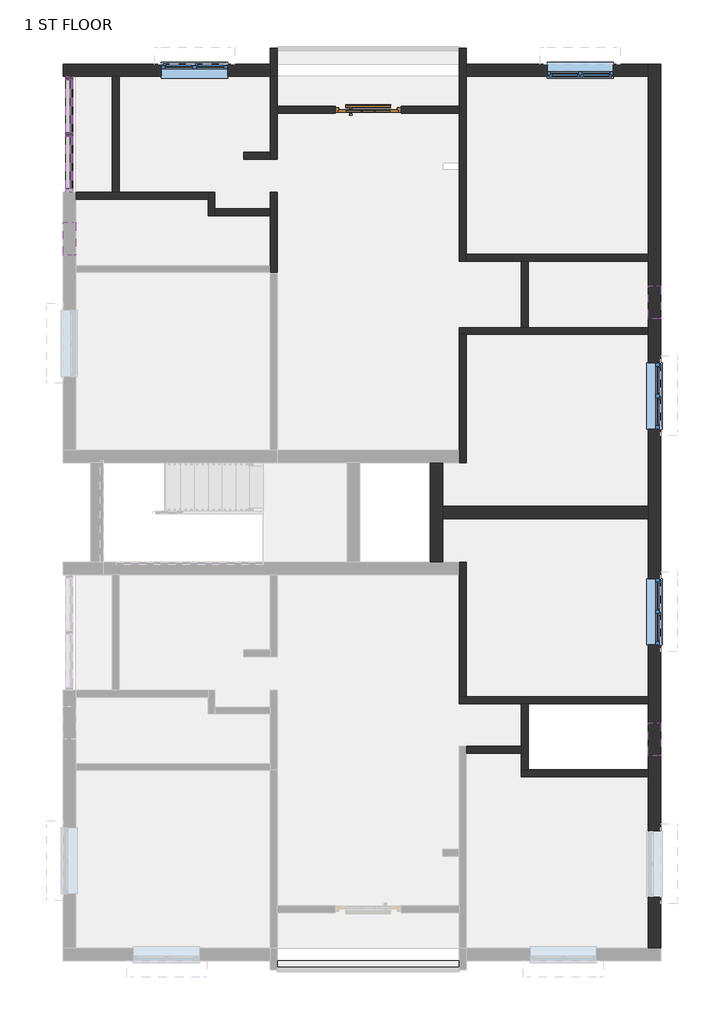
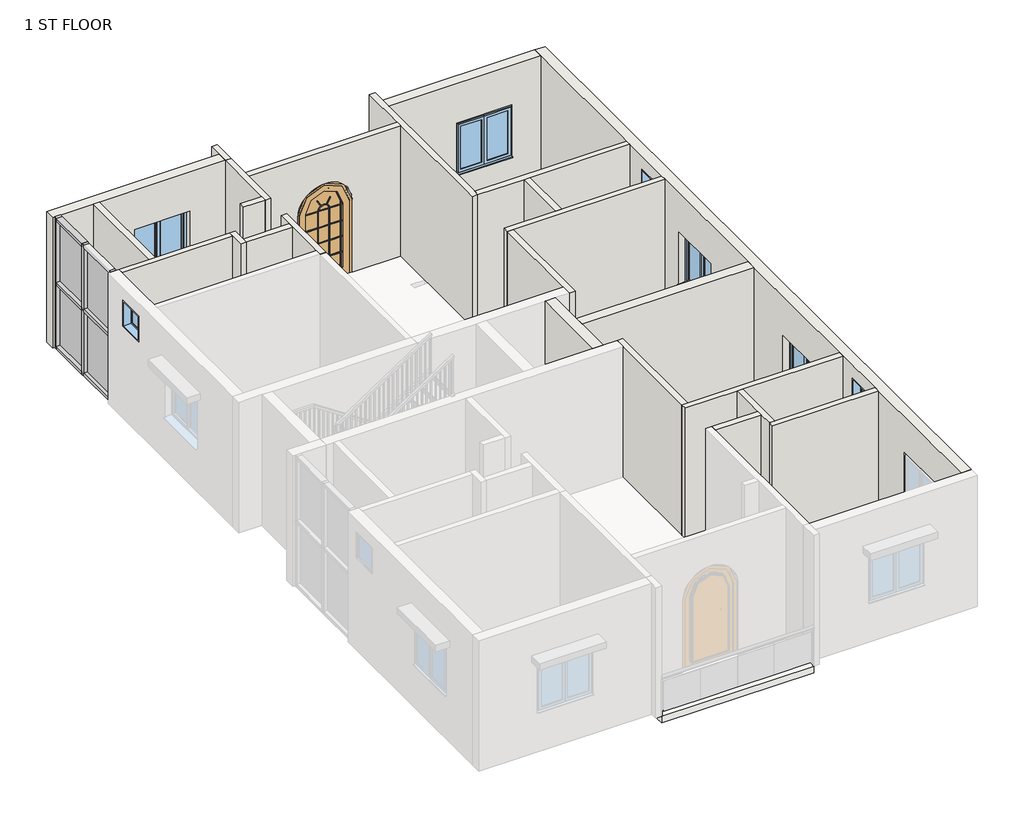
# One storey, part 2 of 4: 24 walls, 10 members, 7 windows, 4 plates, 1 door, 1 slab.
"""IFC4 building model written with IfcOpenShell, lengths in millimetres."""

from ifc_helpers import new_model, si_unit, point, frame, frame_2d, origin, place, context, project, spatial, polyline, circle_curve, trimmed, segment, composite_curve, outline, extrude, faceted_brep, transform, mapped, element, save
from components import door_arched_single_french_glass_wood_exterior_4_x_7_french_5c4dec95, member_801a2072, member_82905deb, member_88aa5c81, member_4491d118, system_panel_glazed_a8655be6, window_80340324, w2_windows_4_x_4_9dec5fc7

model = new_model("IFC4")

# Units and contexts
model_context = context("Model", 3, world=origin())
ifc_project = project(units=[si_unit("LENGTHUNIT", "METRE", prefix="MILLI")], contexts=[model_context])

# Site, building, storey
site = spatial("IfcSite", under=ifc_project)
building = spatial("IfcBuilding", under=site)
storey = spatial("IfcBuildingStorey", under=building, Name="1 ST FLOOR", Elevation=6096.0)

# Door
placement = place(None, origin())
door_arched_single_french_glass_wood_exterior_4_x_7_french_shape = door_arched_single_french_glass_wood_exterior_4_x_7_french_5c4dec95(model_context)
element("IfcDoor", 1, ObjectType="Door_Arched_Single_French_Glass_Wood_Exterior : 4' x 7' french door", at=placement, inside=storey, context=model_context, shape_type="MappedRepresentation", body=[
    mapped(door_arched_single_french_glass_wood_exterior_4_x_7_french_shape, transform((-817.6012202, 12433.0309003, 6096.0), x_axis=(1.0, 0.0, 0.0), y_axis=(0.0, 1.0, 0.0), z_axis=(0.0, 0.0, 1.0))),
])

# Members
member_shape = member_801a2072(model_context)
element("IfcMember", 2, ObjectType="Rectangular Mullion : 2.5\" x 5\" rectangular", at=placement, inside=storey, context=model_context, shape_type="MappedRepresentation", body=[
    mapped(member_shape, transform((-6318.2887202, 12007.5809003, 9144.0), x_axis=(0.0, 0.0, 1.0), y_axis=(-1.0, 0.0, 0.0), z_axis=(0.0, -1.0, 0.0))),
])
element("IfcMember", 3, ObjectType="Rectangular Mullion : 2.5\" x 5\" rectangular", at=placement, inside=storey, context=model_context, shape_type="MappedRepresentation", body=[
    mapped(member_shape, transform((-6318.2887202, 12979.1309003, 6096.0), x_axis=(0.0, 0.0, -1.0), y_axis=(-1.0, 0.0, 0.0), z_axis=(0.0, 1.0, 0.0))),
])
element("IfcMember", 4, ObjectType="Rectangular Mullion : 2.5\" x 5\" rectangular", at=placement, inside=storey, context=model_context, shape_type="MappedRepresentation", body=[
    mapped(member_shape, transform((-6318.2887202, 11944.0809003, 6096.0), x_axis=(0.0, 0.0, -1.0), y_axis=(-1.0, 0.0, 0.0), z_axis=(0.0, 1.0, 0.0))),
])
member_2_shape = member_82905deb(model_context)
element("IfcMember", 5, ObjectType="Rectangular Mullion : 2.5\" x 5\" rectangular", at=placement, inside=storey, context=model_context, shape_type="MappedRepresentation", body=[
    mapped(member_2_shape, transform((-6318.2887202, 11975.8309003, 6096.0), x_axis=(0.0, -1.0, 0.0), y_axis=(-1.0, 0.0, 0.0), z_axis=(0.0, 0.0, -1.0))),
])
member_3_shape = member_88aa5c81(model_context)
element("IfcMember", 6, ObjectType="Rectangular Mullion : 2.5\" x 5\" rectangular", at=placement, inside=storey, context=model_context, shape_type="MappedRepresentation", body=[
    mapped(member_3_shape, transform((-6318.2887202, 12007.5809003, 7620.0), x_axis=(0.0, 0.0, 1.0), y_axis=(-1.0, 0.0, 0.0), z_axis=(0.0, -1.0, 0.0))),
])
element("IfcMember", 7, ObjectType="Rectangular Mullion : 2.5\" x 5\" rectangular", at=placement, inside=storey, context=model_context, shape_type="MappedRepresentation", body=[
    mapped(member_3_shape, transform((-6318.2887202, 10972.5309003, 7620.0), x_axis=(0.0, 0.0, 1.0), y_axis=(-1.0, 0.0, 0.0), z_axis=(0.0, -1.0, 0.0))),
])
element("IfcMember", 8, ObjectType="Rectangular Mullion : 2.5\" x 5\" rectangular", at=placement, inside=storey, context=model_context, shape_type="MappedRepresentation", body=[
    mapped(member_2_shape, transform((-6318.2887202, 11975.8309003, 7620.0), x_axis=(0.0, -1.0, 0.0), y_axis=(-1.0, 0.0, 0.0), z_axis=(0.0, 0.0, -1.0))),
])
member_4_shape = member_4491d118(model_context)
element("IfcMember", 9, ObjectType="Rectangular Mullion : 2.5\" x 5\" rectangular", at=placement, inside=storey, context=model_context, shape_type="MappedRepresentation", body=[
    mapped(member_4_shape, transform((-6318.2887202, 13042.6309003, 9144.0), x_axis=(0.0, 1.0, 0.0), y_axis=(-1.0, 0.0, 0.0), z_axis=(0.0, 0.0, 1.0))),
])
element("IfcMember", 10, ObjectType="Rectangular Mullion : 2.5\" x 5\" rectangular", at=placement, inside=storey, context=model_context, shape_type="MappedRepresentation", body=[
    mapped(member_4_shape, transform((-6318.2887202, 10909.0309003, 7620.0), x_axis=(0.0, -1.0, 0.0), y_axis=(-1.0, 0.0, 0.0), z_axis=(0.0, 0.0, -1.0))),
])
element("IfcMember", 11, ObjectType="Rectangular Mullion : 2.5\" x 5\" rectangular", at=placement, inside=storey, context=model_context, shape_type="MappedRepresentation", body=[
    mapped(member_4_shape, transform((-6318.2887202, 13042.6309003, 7620.0), x_axis=(0.0, 1.0, 0.0), y_axis=(-1.0, 0.0, 0.0), z_axis=(0.0, 0.0, 1.0))),
])

# Plates
system_panel_glazed_shape = system_panel_glazed_a8655be6(model_context)
element("IfcPlate", 12, ObjectType="System Panel : Glazed", at=placement, inside=storey, context=model_context, shape_type="MappedRepresentation", body=[
    mapped(system_panel_glazed_shape, transform((-6318.2887202, 12493.3559003, 6159.5), x_axis=(0.0, -1.0, 0.0), y_axis=(1.0, 0.0, 0.0), z_axis=(0.0, 0.0, 1.0))),
])
element("IfcPlate", 13, ObjectType="System Panel : Glazed", at=placement, inside=storey, context=model_context, shape_type="MappedRepresentation", body=[
    mapped(system_panel_glazed_shape, transform((-6318.2887202, 11458.3059003, 6159.5), x_axis=(0.0, -1.0, 0.0), y_axis=(1.0, 0.0, 0.0), z_axis=(0.0, 0.0, 1.0))),
])
element("IfcPlate", 14, ObjectType="System Panel : Glazed", at=placement, inside=storey, context=model_context, shape_type="MappedRepresentation", body=[
    mapped(system_panel_glazed_shape, transform((-6318.2887202, 12493.3559003, 7651.75), x_axis=(0.0, -1.0, 0.0), y_axis=(1.0, 0.0, 0.0), z_axis=(0.0, 0.0, 1.0))),
])
element("IfcPlate", 15, ObjectType="System Panel : Glazed", at=placement, inside=storey, context=model_context, shape_type="MappedRepresentation", body=[
    mapped(system_panel_glazed_shape, transform((-6318.2887202, 11458.3059003, 7651.75), x_axis=(0.0, -1.0, 0.0), y_axis=(1.0, 0.0, 0.0), z_axis=(0.0, 0.0, 1.0))),
])

# Slab
element("IfcSlab", 16, ObjectType="bathroom tiles", at=placement, inside=storey, context=model_context, shape_type="SweptSolid", body=[
    extrude(outline(polyline([(858.7987798, -3238.7690997), (858.7987798, -3403.8690997), (-2494.0012202, -3403.8690997), (-2494.0012202, -3238.7690997), (858.7987798, -3238.7690997)])), frame((0.0, 0.0, 5943.6), z_axis=(0.0, 0.0, 1.0), x_axis=(1.0, 0.0, 0.0)), (0.0, 0.0, 1.0), 152.4),
])

# Walls
element("IfcWall", 17, ObjectType="OUTER WALL 9\"", at=placement, inside=storey, context=model_context, shape_type="Brep", body=[
    faceted_brep([(4567.1987798, -3010.1690997, 6096.0), (4567.1987798, 13271.2309003, 6096.0), (4567.1987798, 13271.2309003, 9144.0), (4567.1987798, -3010.1690997, 9144.0), (4567.1987798, -844.8190997, 7096.0), (4567.1987798, -2064.0190997, 7096.0), (4567.1987798, -2064.0190997, 8315.2), (4567.1987798, -844.8190997, 8315.2), (4567.1987798, 2577.8309003, 7010.4), (4567.1987798, 2577.8309003, 8229.6), (4567.1987798, 3797.0309003, 8229.6), (4567.1987798, 3797.0309003, 7010.4), (4567.1987798, 6552.9309003, 7010.4), (4567.1987798, 6552.9309003, 8229.6), (4567.1987798, 7772.1309003, 8229.6), (4567.1987798, 7772.1309003, 7010.4), (4567.1987798, 539.4809003, 8839.2), (4567.1987798, 1149.0809003, 8839.2), (4567.1987798, 1149.0809003, 8229.6), (4567.1987798, 539.4809003, 8229.6), (4567.1987798, 8584.9309003, 8839.2), (4567.1987798, 9194.5309003, 8839.2), (4567.1987798, 9194.5309003, 8229.6), (4567.1987798, 8584.9309003, 8229.6), (4338.5987798, -3010.1690997, 6096.0), (4338.5987798, -3010.1690997, 9144.0), (4338.5987798, 152.1309003, 9144.0), (4338.5987798, 279.1309003, 9144.0), (4338.5987798, 1498.3309003, 9144.0), (4338.5987798, 1625.3309003, 9144.0), (4338.5987798, 4901.9309003, 9144.0), (4338.5987798, 5130.5309003, 9144.0), (4338.5987798, 8292.8309003, 9144.0), (4338.5987798, 8419.8309003, 9144.0), (4338.5987798, 9639.0309003, 9144.0), (4338.5987798, 9766.0309003, 9144.0), (4338.5987798, 13042.6309003, 9144.0), (4338.5987798, 13271.2309003, 9144.0), (4338.5987798, 13271.2309003, 6096.0), (4338.5987798, 13042.6309003, 6096.0), (4338.5987798, 9766.0309003, 6096.0), (4338.5987798, 9639.0309003, 6096.0), (4338.5987798, 8419.8309003, 6096.0), (4338.5987798, 8292.8309003, 6096.0), (4338.5987798, 5130.5309003, 6096.0), (4338.5987798, 4901.9309003, 6096.0), (4338.5987798, 1625.3309003, 6096.0), (4338.5987798, 1498.3309003, 6096.0), (4338.5987798, 279.1309003, 6096.0), (4338.5987798, 152.1309003, 6096.0), (4338.5987798, -844.8190997, 7096.0), (4338.5987798, -844.8190997, 8315.2), (4338.5987798, -2064.0190997, 8315.2), (4338.5987798, -2064.0190997, 7096.0), (4338.5987798, 2577.8309003, 7010.4), (4338.5987798, 3797.0309003, 7010.4), (4338.5987798, 3797.0309003, 8229.6), (4338.5987798, 2577.8309003, 8229.6), (4338.5987798, 6552.9309003, 7010.4), (4338.5987798, 7772.1309003, 7010.4), (4338.5987798, 7772.1309003, 8229.6), (4338.5987798, 6552.9309003, 8229.6), (4338.5987798, 539.4809003, 8839.2), (4338.5987798, 539.4809003, 8229.6), (4338.5987798, 1149.0809003, 8229.6), (4338.5987798, 1149.0809003, 8839.2), (4338.5987798, 8584.9309003, 8839.2), (4338.5987798, 8584.9309003, 8229.6), (4338.5987798, 9194.5309003, 8229.6), (4338.5987798, 9194.5309003, 8839.2)], [[[0, 1, 2, 3], [4, 5, 6, 7], [8, 9, 10, 11], [12, 13, 14, 15], [16, 17, 18, 19], [20, 21, 22, 23]], [[24, 25, 26, 27, 28, 29, 30, 31, 32, 33, 34, 35, 36, 37, 38, 39, 40, 41, 42, 43, 44, 45, 46, 47, 48, 49], [50, 51, 52, 53], [54, 55, 56, 57], [58, 59, 60, 61], [62, 63, 64, 65], [66, 67, 68, 69]], [[1, 0, 24, 49, 48, 47, 46, 45, 44, 43, 42, 41, 40, 39, 38]], [[3, 2, 37, 36, 35, 34, 33, 32, 31, 30, 29, 28, 27, 26, 25]], [[0, 3, 25, 24]], [[2, 1, 38, 37]], [[51, 50, 4, 7]], [[52, 51, 7, 6]], [[53, 52, 6, 5]], [[50, 53, 5, 4]], [[9, 8, 54, 57]], [[10, 9, 57, 56]], [[11, 10, 56, 55]], [[8, 11, 55, 54]], [[13, 12, 58, 61]], [[14, 13, 61, 60]], [[15, 14, 60, 59]], [[12, 15, 59, 58]], [[63, 62, 16, 19]], [[64, 63, 19, 18]], [[65, 64, 18, 17]], [[62, 65, 17, 16]], [[67, 66, 20, 23]], [[68, 67, 23, 22]], [[69, 68, 22, 21]], [[66, 69, 21, 20]]]),
])
element("IfcWall", 18, ObjectType="OUTER WALL 9\"", at=placement, inside=storey, context=model_context, shape_type="SweptSolid", body=[
    extrude(outline(polyline([(6096.0, 4338.5987798), (9144.0, 4338.5987798), (9144.0, 985.7987798), (6096.0, 985.7987798), (6096.0, 4338.5987798)]), holes=[polyline([(7010.4, 2479.7847416), (8229.6, 2479.7847416), (8229.6, 3698.9847416), (7010.4, 3698.9847416), (7010.4, 2479.7847416)])]), frame((0.0, 13042.6309003, 0.0), z_axis=(0.0, 1.0, 0.0), x_axis=(0.0, 0.0, 1.0)), (0.0, 0.0, 1.0), 228.6),
])
element("IfcWall", 19, ObjectType="OUTER WALL 9\"", at=placement, inside=storey, context=model_context, shape_type="Brep", body=[
    faceted_brep([(-2621.0012202, 13271.2309003, 6096.0), (-6432.5887202, 13271.2309003, 6096.0), (-6432.5887202, 13271.2309003, 9144.0), (-2621.0012202, 13271.2309003, 9144.0), (-3402.0512202, 13271.2309003, 7010.4), (-3402.0512202, 13271.2309003, 8229.6), (-4621.2512202, 13271.2309003, 8229.6), (-4621.2512202, 13271.2309003, 7010.4), (-2621.0012202, 13042.6309003, 6096.0), (-2621.0012202, 13042.6309003, 9144.0), (-5402.3012202, 13042.6309003, 9144.0), (-5529.3012202, 13042.6309003, 9144.0), (-6432.5887202, 13042.6309003, 9144.0), (-6432.5887202, 13042.6309003, 6096.0), (-5529.3012202, 13042.6309003, 6096.0), (-5402.3012202, 13042.6309003, 6096.0), (-3402.0512202, 13042.6309003, 7010.4), (-4621.2512202, 13042.6309003, 7010.4), (-4621.2512202, 13042.6309003, 8229.6), (-3402.0512202, 13042.6309003, 8229.6)], [[[0, 1, 2, 3], [4, 5, 6, 7]], [[8, 9, 10, 11, 12, 13, 14, 15], [16, 17, 18, 19]], [[1, 0, 8, 15, 14, 13]], [[3, 2, 12, 11, 10, 9]], [[2, 1, 13, 12]], [[5, 4, 16, 19]], [[6, 5, 19, 18]], [[7, 6, 18, 17]], [[4, 7, 17, 16]], [[0, 3, 9, 8]]]),
])
element("IfcWall", 20, ObjectType="OUTER WALL 9\"", at=placement, inside=storey, context=model_context, shape_type="Brep", body=[
    faceted_brep([(553.9987798, 4101.8309003, 6096.0), (553.9987798, 4901.9309003, 6096.0), (553.9987798, 5130.5309003, 6096.0), (553.9987798, 5930.6309003, 6096.0), (553.9987798, 5930.6309003, 9144.0), (553.9987798, 5130.5309003, 9144.0), (553.9987798, 4901.9309003, 9144.0), (553.9987798, 4101.8309003, 9144.0), (325.3987798, 4101.8309003, 6096.0), (325.3987798, 4101.8309003, 9144.0), (325.3987798, 5930.6309003, 9144.0), (325.3987798, 5930.6309003, 6096.0)], [[[0, 1, 2, 3, 4, 5, 6, 7]], [[8, 9, 10, 11]], [[3, 2, 1, 0, 8, 11]], [[7, 6, 5, 4, 10, 9]], [[0, 7, 9, 8]], [[4, 3, 11, 10]]]),
])
element("IfcWall", 21, ObjectType="OUTER WALL 9\"", at=placement, inside=storey, context=model_context, shape_type="SweptSolid", body=[
    extrude(outline(polyline([(4338.5987798, 4901.9309003), (553.9987798, 4901.9309003), (553.9987798, 5130.5309003), (4338.5987798, 5130.5309003), (4338.5987798, 4901.9309003)])), frame((0.0, 0.0, 6096.0), z_axis=(0.0, 0.0, 1.0), x_axis=(1.0, 0.0, 0.0)), (0.0, 0.0, 1.0), 3048.0),
])
element("IfcWall", 22, ObjectType="inner wall 5\"", at=placement, inside=storey, context=model_context, shape_type="SweptSolid", body=[
    extrude(outline(polyline([(-5529.3012202, 10909.0309003), (-5529.3012202, 13042.6309003), (-5402.3012202, 13042.6309003), (-5402.3012202, 10909.0309003), (-5529.3012202, 10909.0309003)])), frame((0.0, 0.0, 6096.0), z_axis=(0.0, 0.0, 1.0), x_axis=(1.0, 0.0, 0.0)), (0.0, 0.0, 1.0), 3048.0),
])
element("IfcWall", 23, ObjectType="inner wall 5\"", at=placement, inside=storey, context=model_context, shape_type="Brep", body=[
    faceted_brep([(-2621.0012202, 13042.6309003, 6096.0), (-2621.0012202, 11645.6309003, 6096.0), (-2621.0012202, 11518.6309003, 6096.0), (-2621.0012202, 11518.6309003, 9144.0), (-2621.0012202, 11645.6309003, 9144.0), (-2621.0012202, 13042.6309003, 9144.0), (-2494.0012202, 13042.6309003, 6096.0), (-2494.0012202, 13042.6309003, 9144.0), (-2494.0012202, 12496.5309003, 9144.0), (-2494.0012202, 12369.5309003, 9144.0), (-2494.0012202, 11518.6309003, 9144.0), (-2494.0012202, 11518.6309003, 6096.0), (-2494.0012202, 12369.5309003, 6096.0), (-2494.0012202, 12496.5309003, 6096.0)], [[[0, 1, 2, 3, 4, 5]], [[6, 7, 8, 9, 10, 11, 12, 13]], [[2, 1, 0, 6, 13, 12, 11]], [[5, 4, 3, 10, 9, 8, 7]], [[3, 2, 11, 10]], [[0, 5, 7, 6]]]),
])
element("IfcWall", 24, ObjectType="inner wall 5\"", at=placement, inside=storey, context=model_context, shape_type="SweptSolid", body=[
    extrude(outline(polyline([(-3103.6012202, 11645.6309003), (-2621.0012202, 11645.6309003), (-2621.0012202, 11518.6309003), (-3103.6012202, 11518.6309003), (-3103.6012202, 11645.6309003)])), frame((0.0, 0.0, 6096.0), z_axis=(0.0, 0.0, 1.0), x_axis=(1.0, 0.0, 0.0)), (0.0, 0.0, 1.0), 3048.0),
])
element("IfcWall", 25, ObjectType="inner wall 5\"", at=placement, inside=storey, context=model_context, shape_type="Brep", body=[
    faceted_brep([(-6202.4012202, 10782.0309003, 6096.0), (-3764.0012202, 10782.0309003, 6096.0), (-3764.0012202, 10782.0309003, 9144.0), (-6202.4012202, 10782.0309003, 9144.0), (-6202.4012202, 10909.0309003, 6096.0), (-6202.4012202, 10909.0309003, 9144.0), (-5529.3012202, 10909.0309003, 9144.0), (-5402.3012202, 10909.0309003, 9144.0), (-3764.0012202, 10909.0309003, 9144.0), (-3764.0012202, 10909.0309003, 6096.0), (-5402.3012202, 10909.0309003, 6096.0), (-5529.3012202, 10909.0309003, 6096.0)], [[[0, 1, 2, 3]], [[4, 5, 6, 7, 8, 9, 10, 11]], [[1, 0, 4, 11, 10, 9]], [[3, 2, 8, 7, 6, 5]], [[0, 3, 5, 4]], [[2, 1, 9, 8]]]),
])
element("IfcWall", 26, ObjectType="inner wall 5\"", at=placement, inside=storey, context=model_context, shape_type="Brep", body=[
    faceted_brep([(-3764.0012202, 10909.0309003, 6096.0), (-3764.0012202, 10782.0309003, 6096.0), (-3764.0012202, 10477.2309003, 6096.0), (-3764.0012202, 10477.2309003, 9144.0), (-3764.0012202, 10782.0309003, 9144.0), (-3764.0012202, 10909.0309003, 9144.0), (-3637.0012202, 10909.0309003, 6096.0), (-3637.0012202, 10909.0309003, 9144.0), (-3637.0012202, 10604.2309003, 9144.0), (-3637.0012202, 10477.2309003, 9144.0), (-3637.0012202, 10477.2309003, 6096.0), (-3637.0012202, 10604.2309003, 6096.0)], [[[0, 1, 2, 3, 4, 5]], [[6, 7, 8, 9, 10, 11]], [[2, 1, 0, 6, 11, 10]], [[5, 4, 3, 9, 8, 7]], [[0, 5, 7, 6]], [[3, 2, 10, 9]]]),
])
element("IfcWall", 27, ObjectType="inner wall 5\"", at=placement, inside=storey, context=model_context, shape_type="SweptSolid", body=[
    extrude(outline(polyline([(-2621.0012202, 10477.2309003), (-3637.0012202, 10477.2309003), (-3637.0012202, 10604.2309003), (-2621.0012202, 10604.2309003), (-2621.0012202, 10477.2309003)])), frame((0.0, 0.0, 6096.0), z_axis=(0.0, 0.0, 1.0), x_axis=(1.0, 0.0, 0.0)), (0.0, 0.0, 1.0), 3048.0),
])
element("IfcWall", 28, ObjectType="inner wall 5\"", at=placement, inside=storey, context=model_context, shape_type="Brep", body=[
    faceted_brep([(-2621.0012202, 10909.0309003, 6096.0), (-2621.0012202, 10604.2309003, 6096.0), (-2621.0012202, 10477.2309003, 6096.0), (-2621.0012202, 9562.8309003, 6096.0), (-2621.0012202, 9435.8309003, 6096.0), (-2621.0012202, 9435.8309003, 9144.0), (-2621.0012202, 9562.8309003, 9144.0), (-2621.0012202, 10477.2309003, 9144.0), (-2621.0012202, 10604.2309003, 9144.0), (-2621.0012202, 10909.0309003, 9144.0), (-2494.0012202, 10909.0309003, 6096.0), (-2494.0012202, 10909.0309003, 9144.0), (-2494.0012202, 9435.8309003, 9144.0), (-2494.0012202, 9435.8309003, 6096.0)], [[[0, 1, 2, 3, 4, 5, 6, 7, 8, 9]], [[10, 11, 12, 13]], [[4, 3, 2, 1, 0, 10, 13]], [[9, 8, 7, 6, 5, 12, 11]], [[0, 9, 11, 10]], [[5, 4, 13, 12]]]),
])
element("IfcWall", 29, ObjectType="inner wall 5\"", at=placement, inside=storey, context=model_context, shape_type="SweptSolid", body=[
    extrude(outline(polyline([(2001.7987798, 583.9309003), (985.7987798, 583.9309003), (985.7987798, 710.9309003), (2001.7987798, 710.9309003), (2001.7987798, 583.9309003)])), frame((0.0, 0.0, 6096.0), z_axis=(0.0, 0.0, 1.0), x_axis=(1.0, 0.0, 0.0)), (0.0, 0.0, 1.0), 3048.0),
])
element("IfcWall", 30, ObjectType="inner wall 5\"", at=placement, inside=storey, context=model_context, shape_type="Brep", body=[
    faceted_brep([(4338.5987798, 1625.3309003, 6096.0), (985.7987798, 1625.3309003, 6096.0), (858.7987798, 1625.3309003, 6096.0), (858.7987798, 1625.3309003, 9144.0), (985.7987798, 1625.3309003, 9144.0), (4338.5987798, 1625.3309003, 9144.0), (4338.5987798, 1498.3309003, 6096.0), (4338.5987798, 1498.3309003, 9144.0), (2128.7987798, 1498.3309003, 9144.0), (2001.7987798, 1498.3309003, 9144.0), (858.7987798, 1498.3309003, 9144.0), (858.7987798, 1498.3309003, 6096.0), (2001.7987798, 1498.3309003, 6096.0), (2128.7987798, 1498.3309003, 6096.0)], [[[0, 1, 2, 3, 4, 5]], [[6, 7, 8, 9, 10, 11, 12, 13]], [[2, 1, 0, 6, 13, 12, 11]], [[5, 4, 3, 10, 9, 8, 7]], [[3, 2, 11, 10]], [[0, 5, 7, 6]]]),
])
element("IfcWall", 31, ObjectType="inner wall 5\"", at=placement, inside=storey, context=model_context, shape_type="Brep", body=[
    faceted_brep([(985.7987798, 1625.3309003, 6096.0), (985.7987798, 4101.8309003, 6096.0), (985.7987798, 4101.8309003, 9144.0), (985.7987798, 1625.3309003, 9144.0), (858.7987798, 1625.3309003, 6096.0), (858.7987798, 1625.3309003, 9144.0), (858.7987798, 3873.2309003, 9144.0), (858.7987798, 4101.8309003, 9144.0), (858.7987798, 4101.8309003, 6096.0), (858.7987798, 3873.2309003, 6096.0)], [[[0, 1, 2, 3]], [[4, 5, 6, 7, 8, 9]], [[1, 0, 4, 9, 8]], [[3, 2, 7, 6, 5]], [[0, 3, 5, 4]], [[2, 1, 8, 7]]]),
])
element("IfcWall", 32, ObjectType="inner wall 5\"", at=placement, inside=storey, context=model_context, shape_type="Brep", body=[
    faceted_brep([(4338.5987798, 279.1309003, 6096.0), (2128.7987798, 279.1309003, 6096.0), (2001.7987798, 279.1309003, 6096.0), (2001.7987798, 279.1309003, 9144.0), (2128.7987798, 279.1309003, 9144.0), (4338.5987798, 279.1309003, 9144.0), (4338.5987798, 152.1309003, 6096.0), (4338.5987798, 152.1309003, 9144.0), (2001.7987798, 152.1309003, 9144.0), (2001.7987798, 152.1309003, 6096.0)], [[[0, 1, 2, 3, 4, 5]], [[6, 7, 8, 9]], [[2, 1, 0, 6, 9]], [[5, 4, 3, 8, 7]], [[0, 5, 7, 6]], [[3, 2, 9, 8]]]),
])
element("IfcWall", 33, ObjectType="inner wall 5\"", at=placement, inside=storey, context=model_context, shape_type="Brep", body=[
    faceted_brep([(2128.7987798, 279.1309003, 6096.0), (2128.7987798, 1498.3309003, 6096.0), (2128.7987798, 1498.3309003, 9144.0), (2128.7987798, 279.1309003, 9144.0), (2001.7987798, 279.1309003, 6096.0), (2001.7987798, 279.1309003, 9144.0), (2001.7987798, 583.9309003, 9144.0), (2001.7987798, 710.9309003, 9144.0), (2001.7987798, 1498.3309003, 9144.0), (2001.7987798, 1498.3309003, 6096.0), (2001.7987798, 710.9309003, 6096.0), (2001.7987798, 583.9309003, 6096.0)], [[[0, 1, 2, 3]], [[4, 5, 6, 7, 8, 9, 10, 11]], [[1, 0, 4, 11, 10, 9]], [[3, 2, 8, 7, 6, 5]], [[0, 3, 5, 4]], [[2, 1, 9, 8]]]),
])
element("IfcWall", 34, ObjectType="inner wall 5\"", at=placement, inside=storey, context=model_context, shape_type="SweptSolid", body=[
    extrude(outline(composite_curve([segment(polyline([(7774.6, -208.0012202), (6096.0, -208.0012202), (6096.0, 858.7987798), (9144.0, 858.7987798), (9144.0, -2494.0012202), (6096.0, -2494.0012202), (6096.0, -1427.2012202), (7774.6, -1427.2012202)]), True, "CONTINUOUS"), segment(trimmed(circle_curve(frame_2d((7774.6, -817.6012202)), 609.6), [point((7774.6, -1427.2012202))], [point((7774.6, -208.0012202))], True, "CARTESIAN"), True, "CONTINUOUS")], self_intersect=False)), frame((0.0, 12369.5309003, 0.0), z_axis=(0.0, 1.0, 0.0), x_axis=(0.0, 0.0, 1.0)), (0.0, 0.0, 1.0), 127.0),
])
element("IfcWall", 35, ObjectType="inner wall 5\"", at=placement, inside=storey, context=model_context, shape_type="Brep", body=[
    faceted_brep([(858.7987798, 13563.3309003, 6096.0), (858.7987798, 12496.5309003, 6096.0), (858.7987798, 12369.5309003, 6096.0), (858.7987798, 9639.0309003, 6096.0), (858.7987798, 9639.0309003, 9144.0), (858.7987798, 12369.5309003, 9144.0), (858.7987798, 12496.5309003, 9144.0), (858.7987798, 13563.3309003, 9144.0), (985.7987798, 13563.3309003, 6096.0), (985.7987798, 13563.3309003, 9144.0), (985.7987798, 13271.2309003, 9144.0), (985.7987798, 13042.6309003, 9144.0), (985.7987798, 9766.0309003, 9144.0), (985.7987798, 9639.0309003, 9144.0), (985.7987798, 9639.0309003, 6096.0), (985.7987798, 9766.0309003, 6096.0), (985.7987798, 13042.6309003, 6096.0), (985.7987798, 13271.2309003, 6096.0)], [[[0, 1, 2, 3, 4, 5, 6, 7]], [[8, 9, 10, 11, 12, 13, 14, 15, 16, 17]], [[3, 2, 1, 0, 8, 17, 16, 15, 14]], [[7, 6, 5, 4, 13, 12, 11, 10, 9]], [[0, 7, 9, 8]], [[4, 3, 14, 13]]]),
])
element("IfcWall", 36, ObjectType="inner wall 5\"", at=placement, inside=storey, context=model_context, shape_type="Brep", body=[
    faceted_brep([(4338.5987798, 9766.0309003, 6096.0), (985.7987798, 9766.0309003, 6096.0), (985.7987798, 9766.0309003, 9144.0), (4338.5987798, 9766.0309003, 9144.0), (4338.5987798, 9639.0309003, 6096.0), (4338.5987798, 9639.0309003, 9144.0), (2128.7987798, 9639.0309003, 9144.0), (2001.7987798, 9639.0309003, 9144.0), (985.7987798, 9639.0309003, 9144.0), (985.7987798, 9639.0309003, 6096.0), (2001.7987798, 9639.0309003, 6096.0), (2128.7987798, 9639.0309003, 6096.0)], [[[0, 1, 2, 3]], [[4, 5, 6, 7, 8, 9, 10, 11]], [[1, 0, 4, 11, 10, 9]], [[3, 2, 8, 7, 6, 5]], [[0, 3, 5, 4]], [[2, 1, 9, 8]]]),
])
element("IfcWall", 37, ObjectType="inner wall 5\"", at=placement, inside=storey, context=model_context, shape_type="Brep", body=[
    faceted_brep([(4338.5987798, 8419.8309003, 6096.0), (2128.7987798, 8419.8309003, 6096.0), (2001.7987798, 8419.8309003, 6096.0), (858.7987798, 8419.8309003, 6096.0), (858.7987798, 8419.8309003, 9144.0), (2001.7987798, 8419.8309003, 9144.0), (2128.7987798, 8419.8309003, 9144.0), (4338.5987798, 8419.8309003, 9144.0), (4338.5987798, 8292.8309003, 6096.0), (4338.5987798, 8292.8309003, 9144.0), (985.7987798, 8292.8309003, 9144.0), (858.7987798, 8292.8309003, 9144.0), (858.7987798, 8292.8309003, 6096.0), (985.7987798, 8292.8309003, 6096.0)], [[[0, 1, 2, 3, 4, 5, 6, 7]], [[8, 9, 10, 11, 12, 13]], [[3, 2, 1, 0, 8, 13, 12]], [[7, 6, 5, 4, 11, 10, 9]], [[0, 7, 9, 8]], [[4, 3, 12, 11]]]),
])
element("IfcWall", 38, ObjectType="inner wall 5\"", at=placement, inside=storey, context=model_context, shape_type="SweptSolid", body=[
    extrude(outline(polyline([(2128.7987798, 9639.0309003), (2128.7987798, 8419.8309003), (2001.7987798, 8419.8309003), (2001.7987798, 9639.0309003), (2128.7987798, 9639.0309003)])), frame((0.0, 0.0, 6096.0), z_axis=(0.0, 0.0, 1.0), x_axis=(1.0, 0.0, 0.0)), (0.0, 0.0, 1.0), 3048.0),
])
element("IfcWall", 39, ObjectType="inner wall 5\"", at=placement, inside=storey, context=model_context, shape_type="Brep", body=[
    faceted_brep([(858.7987798, 8292.8309003, 6096.0), (858.7987798, 6159.2309003, 6096.0), (858.7987798, 5930.6309003, 6096.0), (858.7987798, 5930.6309003, 9144.0), (858.7987798, 6159.2309003, 9144.0), (858.7987798, 8292.8309003, 9144.0), (985.7987798, 8292.8309003, 6096.0), (985.7987798, 8292.8309003, 9144.0), (985.7987798, 5930.6309003, 9144.0), (985.7987798, 5930.6309003, 6096.0)], [[[0, 1, 2, 3, 4, 5]], [[6, 7, 8, 9]], [[2, 1, 0, 6, 9]], [[5, 4, 3, 8, 7]], [[0, 5, 7, 6]], [[3, 2, 9, 8]]]),
])
element("IfcWall", 40, ObjectType="inner wall 5\"", at=placement, inside=storey, context=model_context, shape_type="Brep", body=[
    faceted_brep([(-2494.0012202, 13042.6309003, 6096.0), (-2494.0012202, 13563.3309003, 6096.0), (-2494.0012202, 13563.3309003, 9144.0), (-2494.0012202, 13042.6309003, 9144.0), (-2621.0012202, 13042.6309003, 6096.0), (-2621.0012202, 13042.6309003, 9144.0), (-2621.0012202, 13271.2309003, 9144.0), (-2621.0012202, 13563.3309003, 9144.0), (-2621.0012202, 13563.3309003, 6096.0), (-2621.0012202, 13271.2309003, 6096.0)], [[[0, 1, 2, 3]], [[4, 5, 6, 7, 8, 9]], [[1, 0, 4, 9, 8]], [[2, 1, 8, 7]], [[3, 2, 7, 6, 5]], [[0, 3, 5, 4]]]),
])

# Windows
window_shape = window_80340324(model_context)
element("IfcWindow", 41, ObjectType="Fixed : 24\" x 24\"", at=placement, inside=storey, context=model_context, shape_type="MappedRepresentation", body=[
    mapped(window_shape, transform((4452.8987798, 8851.6309003, 7315.2), x_axis=(0.0, -1.0, 0.0), y_axis=(1.0, 0.0, 0.0), z_axis=(0.0, 0.0, 1.0))),
])
element("IfcWindow", 42, ObjectType="Fixed : 24\" x 24\"", at=placement, inside=storey, context=model_context, shape_type="MappedRepresentation", body=[
    mapped(window_shape, transform((4452.8987798, 806.1809003, 7315.2), x_axis=(0.0, -1.0, 0.0), y_axis=(1.0, 0.0, 0.0), z_axis=(0.0, 0.0, 1.0))),
])
element("IfcWindow", 43, ObjectType="Fixed : 24\" x 24\"", at=placement, inside=storey, context=model_context, shape_type="MappedRepresentation", body=[
    mapped(window_shape, transform((-6318.2887202, 10020.0309003, 7315.2), x_axis=(0.0, -1.0, 0.0), y_axis=(1.0, 0.0, 0.0), z_axis=(0.0, 0.0, 1.0))),
])
w2_windows_4_x_4_shape = w2_windows_4_x_4_9dec5fc7(model_context)
element("IfcWindow", 44, ObjectType="w2 : windows 4' x 4'", at=placement, inside=storey, context=model_context, shape_type="MappedRepresentation", body=[
    mapped(w2_windows_4_x_4_shape, transform((3089.3847416, 13156.9309003, 6010.4), x_axis=(1.0, 0.0, 0.0), y_axis=(0.0, 1.0, 0.0), z_axis=(0.0, 0.0, 1.0))),
])
element("IfcWindow", 45, ObjectType="w2 : windows 4' x 4'", at=placement, inside=storey, context=model_context, shape_type="MappedRepresentation", body=[
    mapped(w2_windows_4_x_4_shape, transform((-4011.6512202, 13156.9309003, 6010.4), x_axis=(-1.0, 0.0, 0.0), y_axis=(0.0, -1.0, 0.0), z_axis=(0.0, 0.0, 1.0))),
])
element("IfcWindow", 46, ObjectType="w2 : windows 4' x 4'", at=placement, inside=storey, context=model_context, shape_type="MappedRepresentation", body=[
    mapped(w2_windows_4_x_4_shape, transform((4452.8987798, 7162.5309003, 6010.4), x_axis=(0.0, 1.0, 0.0), y_axis=(-1.0, 0.0, 0.0), z_axis=(0.0, 0.0, 1.0))),
])
element("IfcWindow", 47, ObjectType="w2 : windows 4' x 4'", at=placement, inside=storey, context=model_context, shape_type="MappedRepresentation", body=[
    mapped(w2_windows_4_x_4_shape, transform((4452.8987798, 3187.4309003, 6010.4), x_axis=(0.0, 1.0, 0.0), y_axis=(-1.0, 0.0, 0.0), z_axis=(0.0, 0.0, 1.0))),
])

save(model, "model.ifc")

# Revit data of these elements
# Type "Door_Arched_Single_French_Glass_Wood_Exterior : 4' x 7' french door"
#   Type Mark = "17"
#   Type Comments = "External Single"
#   Operation = "SingleSwingRight"
#   Keynote = "L20"
#   Analytic Construction = "<None>"
#   Wrap Layers (Int) from Ext = 0' - 6.98819"
#   Wrap Layers (Ext) from Ext = 0' - 4.03543"
#   Thickness = 0' - 1.73228"
#   Stile Shutting = 0' - 5.90551"
#   Stile - Top Rail = 0' - 5.90551"
#   Stile - Hanging = 0' - 5.90551"
#   Stile - Bottom Rail = 0' - 6.88976"
#   Rough Width = 4' - 0"
#   Rough Height = 7' - 0"
#   O/A Frame Width = 0' - 2.51969"
#   Handle Z Distance = 3' - 5.33858"
#   Glazing Thickness = 0' - 0.94488"
#   Glazing Bar Thickness = 0' - 0.7874"
#   FrameWidth = 0' - 1.65354"
#   FrameOffset - External = 0' - 0.98425"
#   FrameDepth = 0' - 3.50394"
#   Door Panel Width = 3' - 7.94488"
#   Handle X Distance = 0' - 2.95276"
#   Height = 7' - 0"
#   Structural Tolerance = 0' - 0.25591"
#   Tolerance = 0' - 0.11811"
#   Undercut = 0' - 0.15748"
#   Width = 4' - 0"
#   Door Panel Thickness = 0' - 1.73228"
#   Door Panel Height = 6' - 9.81496"
#   Cavity Closer Width = 0' - 1.9685"
#   Cavity Closer Offset from Ext = 0' - 4.03543"
#   Cavity Closer Depth = 0' - 3.34646"
#   Vis - Ironmongery = yes
#   Vis - Cavity Closers = yes
#   Define Thermal Properties by = 1
#   Material Glass = Door - Glazing
#   Handle Style = element 430241
#   Material Door = Door - Panel
#   Material Frame = BROWN
#   Material Ironmongery = Door - Handle
#   Function = (empty or 0)
#   Wall Closure = (empty or 0)
#   Assembly Code = ""
# Type "Rectangular Mullion : 2.5\" x 5\" rectangular"
#   built-in parameter 1007304 = 0.416667 (stored number, unit not read)
#   built-in parameter 1007301 = 0.104167 (stored number, unit not read)
#   built-in parameter 1007300 = 0.104167 (stored number, unit not read)
# Type "System Panel : Glazed"
#   Construction Type Id = "GSP4R"
#   Analytic Construction = "1/8 in Pilkington single glazing"
#   Visual Light Transmittance = 0.9
#   Solar Heat Gain Coefficient = 0.86
#   Heat Transfer Coefficient (U) = 1.18115 BTU/(h·ft²·°F)
#   Define Thermal Properties by = 1
# Type "bathroom tiles"
#   Assembly Code = "B1010"
#   Function = 0
#   Layers, outside or top first: 0' - 6" "tile flooring" (function 1)
# Type "OUTER WALL 9\""
#   Assembly Code = "B2010"
#   Layers, outside or top first: 0' - 9" "ROSE COLOUR" (function 1)
# Type "inner wall 5\""
#   Assembly Code = "B2010"
#   Layers, outside or top first: 0' - 5" "ROSE COLOUR" (function 1)
# Type "Fixed : 24\" x 24\""
#   Type Mark = "3"
#   Construction Type Id = "GSP4R"
#   Assembly Code = "B2020100"
#   Analytic Construction = "1/8 in Pilkington single glazing"
#   Visual Light Transmittance = 0.9
#   Solar Heat Gain Coefficient = 0.78
#   Heat Transfer Coefficient (U) = 0.6496 BTU/(h·ft²·°F)
#   Height = 2' - 0"
#   Default Sill Height = 3' - 0"
#   Width = 2' - 0"
#   Window Inset = 0' - 0 3/4"
#   Define Thermal Properties by = 1
#   Define Thermal Properties by = 1
#   Glass Pane Material = Glass
#   Sash Material = Sash
#   Wall Closure = (empty or 0)
# Type "w2 : windows 4' x 4'"
#   Type Mark = "31"
#   Operation = "DoublePanelVertical"
#   Keynote = "16.05.01"
#   Analytic Construction = "<None>"
#   Rough Width = 4' - 0"
#   Rough Height = 4' - 0"
#   Rahmentiefe = 0' - 2.3622"
#   Rahmenhöhe unten = 0' - 3.14961"
#   Rahmehöhe oben = 0' - 3.14961"
#   Rahmenbreite = 0' - 2.3622"
#   Heat Transfer Coefficient (U) = 2.81836 BTU/(h·ft²·°F)
#   Height = 4' - 0"
#   Flügeltiefe = 0' - 2.3622"
#   Flügelbreite = 0' - 2.3622"
#   Einbautiefe (von außen) [instance default] = 0' - 5.51181"
#   Width = 4' - 0"
#   Kippflügel [instance default] = yes
#   Drehflügel im Grundriß darstellen [instance default] = no
#   Drehflügel [instance default] = yes
#   Define Thermal Properties by = 1
#   Rahmen [instance default] = none
#   Glas [instance default] = blue glass
#   Flügel [instance default] = WINDOW COLOUR WHITE
#   Fensterbank aussen [instance default] = WINDOW COLOUR WHITE
#   Fensterbank innen [instance default] = WINDOW COLOUR WHITE
#   Visual Light Transmittance = 0
#   Thermal Resistance (R) = 0
#   Solar Heat Gain Coefficient = 0
#   Wall Closure = (empty or 0)
# Element 1 (IfcDoor, "Door_Arched_Single_French_Glass_Wood_Exterior : 4' x 7' french door")
#   Phase Created = New Construction
#   Materials on its faces: "Door - Panel", "Door - Handle", "BROWN", "Door - Glazing"
# Elements 2, 3, 4, 5, 6, 7, 8, 9, 10, 11 (IfcMember, "Rectangular Mullion : 2.5\" x 5\" rectangular")
#   Phase Created = New Construction
#   Materials on its faces: "Aluminum"
# Elements 12, 13, 14, 15 (IfcPlate, "System Panel : Glazed")
#   Phase Created = New Construction
#   Materials on its faces: "Glass"
# Element 16 (IfcSlab, "bathroom tiles")
#   Height Offset From Level = 0' - 0"
#   Phase Created = New Construction
#   Materials on its faces: "tile flooring"
# Elements 17, 18, 19, 20, 21 (IfcWall, "OUTER WALL 9\"")
#   Top Offset = 0' - 0"
#   Base Offset = 0' - 0"
#   wall height = 10' - 0"
#   Phase Created = New Construction
#   Base Constraint = 1 ST FLOOR
#   Top Constraint = 2ND FLOOR
#   Materials on its faces: "ROSE COLOUR"
# Elements 22, 23, 24, 25, 26, 27, 28, 29, 30, 31, 32, 33, 34, 35, 36, 37, 38, 39, 40 (IfcWall, "inner wall 5\"")
#   Top Offset = 0' - 0"
#   Base Offset = 0' - 0"
#   wall height = 10' - 0"
#   Phase Created = New Construction
#   Base Constraint = 1 ST FLOOR
#   Top Constraint = 2ND FLOOR
#   Materials on its faces: "ROSE COLOUR"
# Element 41 (IfcWindow, "Fixed : 24\" x 24\"")
#   Mark = "33"
#   Phase Created = New Construction
#   Materials on its faces: "Sash", "Glass"
# Element 42 (IfcWindow, "Fixed : 24\" x 24\"")
#   Mark = "35"
#   Phase Created = New Construction
#   Materials on its faces: "Sash", "Glass"
# Element 43 (IfcWindow, "Fixed : 24\" x 24\"")
#   Mark = "36"
#   Phase Created = New Construction
#   Materials on its faces: "Sash", "Glass"
# Element 44 (IfcWindow, "w2 : windows 4' x 4'")
#   Mark = "24"
#   Phase Created = New Construction
#   Materials on its faces: "WINDOW COLOUR WHITE", "blue glass"
# Element 45 (IfcWindow, "w2 : windows 4' x 4'")
#   Mark = "25"
#   Phase Created = New Construction
#   Materials on its faces: "WINDOW COLOUR WHITE", "blue glass"
# Element 46 (IfcWindow, "w2 : windows 4' x 4'")
#   Mark = "28"
#   Phase Created = New Construction
#   Materials on its faces: "WINDOW COLOUR WHITE", "blue glass"
# Element 47 (IfcWindow, "w2 : windows 4' x 4'")
#   Mark = "29"
#   Phase Created = New Construction
#   Materials on its faces: "WINDOW COLOUR WHITE", "blue glass"
# Materials
#   "Door - Glazing": colour RGB 218 227 224, transparency 0.85
#   "Door - Panel": class "Wood", colour RGB 210 159 95, transparency 0, Cost = 0
#   "BROWN": class "Generic", colour RGB 120 120 120, transparency 0, Cost = 0
#   "Door - Handle": colour RGB 0 0 0, transparency 0, Keynote = "P21"
#   "tile flooring": class "Generic", colour RGB 120 120 120, transparency 0, Cost = 0
#   "ROSE COLOUR": class "Generic", colour RGB 120 120 120, transparency 0, Cost = 0
#   "Glass": class "Glass", colour RGB 0 128 192, transparency 0.75, Description = "Soda Lime Glass", Cost = 0
#   "Sash": class "Wood", colour RGB 224 178 126, transparency 0, Cost = 0
#   "blue glass": class "System", colour RGB 0 0 255, transparency 0.75, Cost = 0
#   "WINDOW COLOUR WHITE": class "Generic", colour RGB 120 120 120, transparency 0, Cost = 0
#   "Aluminum": class "Metal", colour RGB 247 247 247, transparency 0, Description = "Aluminum 6061", Cost = 0
